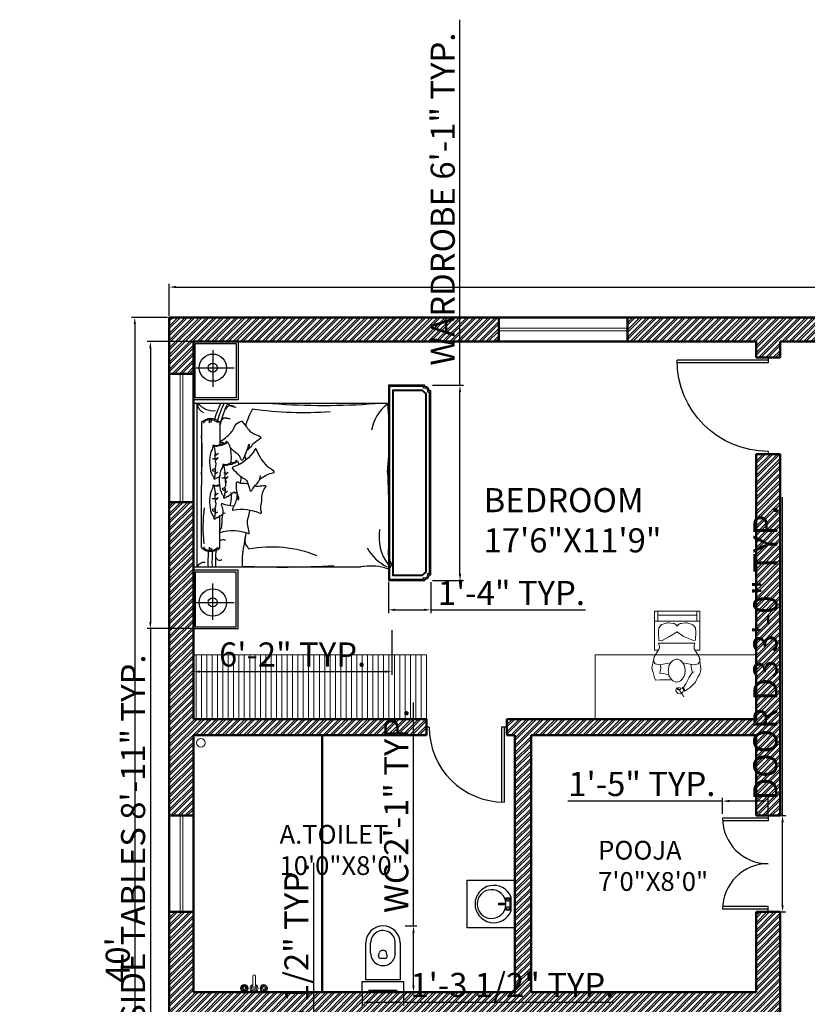
# Model space of a CAD drawing. Units: inches. Extents: x 3590 to 5167, y 65 to 1917.
# Tile 18 of 100: x 3590 to 3884, y 1549 to 1917. Entities that reach past the tile are written whole.
import ezdxf

# ---------------------------------------------------------------- set-up
doc = ezdxf.new("R2010")
doc.units = ezdxf.units.IN
for name, color, linetype, lineweight in [('A-ANNO-DIMS', 2, 'Continuous', 18), ('A-AREA-IDEN', 7, 'Continuous', 18), ('A-DOOR', 3, 'Continuous', 25), ('A-FLOR-FIXT', 8, 'Continuous', 18), ('A-FURN', 21, 'Continuous', 18), ('A-GLAZ', 4, 'Continuous', 18), ('A-WALL', 7, 'Continuous', 50), ('A-WALL-PATT', 251, 'Continuous', 13)]:
    doc.layers.add(name, color=color, linetype=linetype, lineweight=lineweight)
for name, color, linetype in [('FUR', 42, 'Continuous'), ('HA-FUR', 8, 'Continuous'), ('HA-P', 8, 'Continuous'), ('SAN', 5, 'Continuous'), ('SANTEH', 7, 'Continuous'), ('wood', 26, 'Continuous')]:
    doc.layers.add(name, color=color, linetype=linetype)
doc.styles.get("Standard").update_dxf_attribs({"font": 'arial.ttf'})
doc.dimstyles.new('ISO-25', dxfattribs={"dimtxt": 9, "dimasz": 2.5, "dimexe": 1.25, "dimexo": 0.625, "dimtad": 1, "dimdec": 1, "dimlunit": 3, "dimtxsty": 'Standard', "dimcen": 2.5, "dimadec": 0, "dimazin": 0, "dimtfac": 1, "dimtdec": 1, "dimtmove": 0, "dimatfit": 3, "dimfxl": 1, "dimarcsym": 0})

# ---------------------------------------------------------------- blocks, each defined once
blk = doc.blocks.new('*D5')
at = {"layer": 'A-ANNO-DIMS', "color": 0, "lineweight": -2, "transparency": 16777216}
for p, q in [((3645.51, 1806.62), (3645.51, 1818.61)), ((3648.01, 1817.36), (4303.01, 1817.36)), ((4305.51, 1806.62), (4305.51, 1818.61))]:
    blk.add_line(p, q, dxfattribs=at)
at = {"layer": 'A-ANNO-DIMS', "color": 0, "transparency": 16777216}
for points in [[(3648.01, 1817.78), (3648.01, 1816.95), (3645.51, 1817.36)], [(4303.01, 1817.78), (4303.01, 1816.95), (4305.51, 1817.36)]]:
    blk.add_solid(points, dxfattribs=at)
at = {"layer": 'Defpoints', "color": 0, "transparency": 16777216}
for p in [(4305.51, 1817.36), (3645.51, 1806), (4305.51, 1806)]:
    blk.add_point(p, dxfattribs=at)
at = {"layer": 'A-ANNO-DIMS', "color": 0, "transparency": 16777216, "insert": (3975.51, 1822.57), "char_height": 9, "attachment_point": 5}
blk.add_mtext("55'", dxfattribs=at)
blk = doc.blocks.new('*D6')
at = {"layer": 'A-ANNO-DIMS', "color": 0, "lineweight": -2, "transparency": 16777216}
for p, q in [((3644.89, 1806), (3631.39, 1806)), ((3632.64, 1803.5), (3632.64, 1328.5)), ((3644.89, 1326), (3631.39, 1326))]:
    blk.add_line(p, q, dxfattribs=at)
at = {"layer": 'A-ANNO-DIMS', "color": 0, "transparency": 16777216}
for points in [[(3632.22, 1803.5), (3633.06, 1803.5), (3632.64, 1806)], [(3632.22, 1328.5), (3633.06, 1328.5), (3632.64, 1326)]]:
    blk.add_solid(points, dxfattribs=at)
at = {"layer": 'Defpoints', "color": 0, "transparency": 16777216}
for p in [(3645.51, 1806), (3632.64, 1326), (3645.51, 1326)]:
    blk.add_point(p, dxfattribs=at)
at = {"layer": 'A-ANNO-DIMS', "color": 0, "transparency": 16777216, "insert": (3627.42, 1566), "char_height": 9, "attachment_point": 5, "rotation": 90}
blk.add_mtext("40'", dxfattribs=at)
blk = doc.blocks.new('D1')
for p, q in [((1, 0), (1, 34)), ((2, 0), (2, 33.99)), ((0, 0), (2, 0)), ((35, 0), (36, 0))]:
    blk.add_line(p, q)
at = {"ltscale": 0.5}
blk.add_arc((1, 0), 34, 0, 90, dxfattribs=at)
blk = doc.blocks.new('D2')
for p, q in [((1, 0), (1, 28)), ((2, 0), (2, 27.98)), ((0, 0), (2, 0)), ((29, 0), (30, 0))]:
    blk.add_line(p, q)
at = {"ltscale": 0.5}
blk.add_arc((1, 0), 28, 0, 90, dxfattribs=at)
blk = doc.blocks.new('D3')
for p, q in [((1, 0), (1, 17)), ((2, 0), (2, 16.97)), ((34, 0), (34, 16.97)), ((35, 0), (35, 17)), ((0, 0), (2, 0)), ((36, 0), (34, 0))]:
    blk.add_line(p, q)
at = {"ltscale": 0.5}
for centre, start, end in [((1, 0), 0, 90), ((35, 0), 90, 180)]:
    blk.add_arc(centre, 17, start, end, dxfattribs=at)
blk = doc.blocks.new('Faucet - Bathroom top')
for p, q in [((-4.107, 0.125), (-4.375, 0.125)), ((-3.75, 0.4788), (-3.75, 0.75)), ((-3.5, 0.482), (-3.5, 0.75)), ((-3.1461, 0.125), (-2.875, 0.125)), ((3.143, 0.125), (2.875, 0.125)), ((3.5, 0.4788), (3.5, 0.75)), ((3.75, 0.482), (3.75, 0.75)), ((4.1039, 0.125), (4.375, 0.125)), ((-4.1039, -0.125), (-4.375, -0.125)), ((-3.75, -0.4821), (-3.75, -0.75)), ((-3.5, -0.4789), (-3.5, -0.75)), ((-3.143, -0.125), (-2.875, -0.125)), ((-0.5, -0.8639), (-0.5, -4.5)), ((0.5, -4.5), (0.5, -0.8631)), ((3.1461, -0.125), (2.875, -0.125)), ((3.5, -0.4821), (3.5, -0.75)), ((3.75, -0.4789), (3.75, -0.75)), ((4.107, -0.125), (4.375, -0.125))]:
    blk.add_line(p, q)
for centre, radius in [((-3.625, 0), 1.375), ((-4.625, 0), 0.2795), ((-3.625, 0), 0.5), ((-3.625, 1), 0.2795), ((-2.625, 0), 0.2795), ((0, 0), 0.5), ((3.625, 0), 1.375), ((2.625, 0), 0.2795), ((3.625, 0), 0.5), ((3.625, 1), 0.2795), ((4.625, 0), 0.2795), ((-3.625, -1), 0.2795), ((3.625, -1), 0.2795)]:
    blk.add_circle(centre, radius)
for centre, radius, start, end in [((-3.625, 0), 1, 105.2407, 164.2093), ((-3.625, 0), 1, 16.44125, 74.07887), ((0, 0), 1.5, 289.6514, 250.3603), ((0, 0), 1, 300.3431, 239.7554), ((3.625, 0), 1, 106.12, 164.0884), ((3.625, 0), 1, 16.23422, 73.90469), ((-3.625, 0), 1, 196.2342, 253.9047), ((-3.625, 0), 1, 286.12, 344.0884), ((3.625, 0), 1, 196.4413, 254.0789), ((3.625, 0), 1, 285.2407, 344.2093), ((0, -4.5), 0.5, 180, 0)]:
    blk.add_arc(centre, radius, start, end)
blk = doc.blocks.new('y3')
at = {"layer": 'SANTEH', "ltscale": 5}
for p, q in [((38, 131), (38, 521)), ((88, 411), (88, 521)), ((347, 426), (348, 521)), ((398, 521), (398, 131)), ((172, 385), (181, 421)), ((263, 385), (254, 421)), ((244, 358), (191, 358)), ((398, 131), (38, 131)), ((67, 21), (367, 21))]:
    blk.add_line(p, q, dxfattribs=at)
blk.add_lwpolyline([(0, 115), (435, 115), (435, 0), (0, 0), (0, 115)], dxfattribs=at)
for centre, radius, start, end in [((218, 521), 180, 0, 180), ((218, 521), 130, 359.1579, 180), ((218, 411), 130, 180, 5.9855), ((218, 400), 42.2, 30.5234, 149.4766), ((191, 378), 20, 160.5038, 270), ((244, 378), 20, 270, 19.4962)]:
    blk.add_arc(centre, radius, start, end, dxfattribs=at)
blk = doc.blocks.new('r11')
at = {"layer": 'SANTEH', "ltscale": 5}
for p, q in [((0, 0), (600, 0)), ((0, -600), (0, 0)), ((600, 0), (600, -600)), ((210, -50), (390, -50)), ((210, -50), (210, -50)), ((224, -63), (376, -63)), ((224, -113), (224, -63)), ((376, -113), (224, -113)), ((233, -79), (249, -69)), ((233, -98), (233, -79)), ((249, -107), (233, -98)), ((249, -69), (266, -79)), ((266, -98), (249, -107)), ((266, -79), (266, -98)), ((288, -202), (288, -113)), ((312, -113), (312, -202)), ((334, -79), (351, -69)), ((334, -98), (334, -79)), ((351, -107), (334, -98)), ((351, -69), (367, -79)), ((367, -98), (351, -107)), ((367, -79), (367, -98)), ((376, -63), (376, -113)), ((312, -184), (288, -184)), ((312, -202), (288, -202)), ((600, -600), (0, -600))]:
    blk.add_line(p, q, dxfattribs=at)
for centre, radius, start, end in [((300, -266), 234, 112.5, 67.5), ((300, -293), 180, 93.8183, 86.1817)]:
    blk.add_arc(centre, radius, start, end, dxfattribs=at)
blk = doc.blocks.new('A$C0A42580C')
at = {"layer": 'SAN'}
for p, q in [((0.287, 0.03), (0.287, 0.448)), ((2.868, 0.03), (2.868, 0.448)), ((0.095, 0.213), (0.496, 0.213)), ((3.06, 0.213), (2.659, 0.213))]:
    blk.add_line(p, q, dxfattribs=at)
for centre, radius in [((0.287, 0.213), 0.15), ((2.868, 0.213), 0.15), ((0.287, 0.213), 0.05), ((2.868, 0.213), 0.05)]:
    blk.add_circle(centre, radius, dxfattribs=at)
at = {"layer": 'wood'}
for p, q in [((0.678, 0.885), (0.678, 2.139)), ((2.478, 0.802), (2.478, 1.838)), ((2.478, 0), (2.478, 0.802)), ((1.5, 0.342), (1.502, 0.314)), ((1.663, 0.344), (1.643, 0.376)), ((0.888, 0.289), (1.133, 0.289)), ((1.291, 0.235), (1.292, 0.207)), ((1.454, 0.236), (1.434, 0.268)), ((1.729, 0.235), (1.73, 0.207)), ((1.892, 0.236), (1.872, 0.268)), ((2.267, 0.289), (1.916, 0.289)), ((0.678, 0.039), (2.478, 0.039)), ((0.891, 0.089), (1.578, 0.089)), ((2.264, 0.089), (1.578, 0.089)), ((0.678, 0), (2.478, 0))]:
    blk.add_line(p, q, dxfattribs=at)
blk.add_lwpolyline([(0.678, 0), (0.678, 0.885)], dxfattribs=at)
for points in [[(1.516, 0.729, -0.128392), (1.44, 0.883, 0.70791), (1.427, 0.886, -0.16964), (1.185, 0.692, 0.664036), (1.184, 0.678, -0.184649), (1.382, 0.433, 0.662242), (1.397, 0.431, 0.078539), (1.514, 0.567, -0.1736), (1.548, 0.595, -0.02159), (1.636, 0.621, 0.697276), (1.638, 0.641, -0.093019), (1.561, 0.699, 0.216632), (1.472, 0.737, -2.511293)], [(1.68, 0.482, 0.263265), (1.719, 0.484, -0.026108), (1.743, 0.497, 0.027613), (1.714, 0.476, -0.089259), (1.84, 0.429, 0.662242), (1.853, 0.438, -0.162037), (1.888, 0.732, 0.676499), (1.873, 0.748, -0.160513), (1.79, 0.744, 0.07473), (1.72, 0.752, -0.187721), (1.597, 0.796, 0.70791), (1.585, 0.789, -0.010003), (1.592, 0.714, -0.07079), (1.589, 0.672, 0.099539)], [(1.121, 0.345, 0.032543), (1.109, 0.309, -0.658965), (1.092, 0.306, 0.074753), (0.989, 0.423, 0.100988), (0.953, 0.443, -0.270711), (0.875, 0.527, -0.276825), (0.877, 0.534, -0.014937), (0.97, 0.608, 0.134834), (1.013, 0.664, -0.023706), (1.047, 0.737, -0.664036), (1.062, 0.739, -0.035987), (1.119, 0.663, 0.118631), (1.141, 0.641, -0.132738), (1.196, 0.586)], [(1.176, 0.593, 0.013884), (1.155, 0.613, 0.174178), (1.144, 0.618, 0.104076), (1.136, 0.616, 0.389829), (1.132, 0.61, 0.296089), (1.141, 0.602, -0.036701), (1.157, 0.599, -0.040547), (1.302, 0.543, -0.70791), (1.302, 0.53, -0.016811), (1.263, 0.509, 0.11866), (1.241, 0.49, -0.048791), (1.165, 0.405, 0.103757)], [(1.567, 0.601, 0.057807), (1.561, 0.534, -0.173425), (1.546, 0.49, 0.589988), (1.554, 0.471, 0.137312), (1.724, 0.499, 0.137312)], [(1.811, 0.445, -0.069098), (1.783, 0.319, 0.658965), (1.796, 0.306, -0.049789), (1.852, 0.323, -0.103757), (1.89, 0.323, 0.055725), (2.02, 0.31, -0.11866), (2.048, 0.304, 0.016811), (2.088, 0.286, 0.70791), (2.099, 0.294, -0.16964), (2.11, 0.604, 0.664036), (2.1, 0.614, 0.023706), (2.021, 0.597, -0.134834), (1.95, 0.598, 0.012748), (1.852, 0.623)], [(1.311, 0.476, 0.145733), (1.307, 0.468, 0.488583), (1.309, 0.466, -0.012138), (1.313, 0.466, -0.125673), (1.321, 0.465, -0.750706)], [(1.315, 0.475, -0.274893), (1.338, 0.453, 0.051436), (1.347, 0.429, -0.086628), (1.353, 0.408, 0.040196), (1.359, 0.377, -0.184744), (1.356, 0.334, -2.554464)], [(1.317, 0.468, -0.060098), (1.328, 0.457, -0.16247), (1.331, 0.449, 0.120018), (1.349, 0.381, -0.060072), (1.354, 0.369, -0.13107), (1.354, 0.339, -0.024415), (1.353, 0.337, 0.070398), (1.35, 0.323, 0.528689), (1.352, 0.322, -0.069388), (1.356, 0.322, -0.158233), (1.407, 0.306, 0.085461), (1.425, 0.298, 0.147196), (1.657, 0.304, 0.10985), (1.682, 0.319, -0.179095), (1.713, 0.332, -2.318897)], [(1.101, 0.369, 0.145733), (1.097, 0.36, 0.488583), (1.099, 0.358, -0.012138), (1.104, 0.359, -0.125673), (1.112, 0.357, -0.750706)], [(1.106, 0.368, -0.274893), (1.128, 0.345, 0.051436), (1.137, 0.322, -0.086628), (1.144, 0.3, 0.040196), (1.15, 0.27, -0.184744), (1.146, 0.227, -2.554464)], [(1.108, 0.361, -0.060098), (1.119, 0.35, -0.16247), (1.122, 0.341, 0.120018), (1.14, 0.274, -0.060072), (1.145, 0.262, -0.13107), (1.145, 0.232, -0.024415), (1.144, 0.23, 0.070398), (1.141, 0.216, 0.528689), (1.143, 0.214, -0.069388), (1.146, 0.215, -0.158233), (1.198, 0.199, 0.085461), (1.216, 0.191, 0.147196), (1.448, 0.197, 0.10985), (1.473, 0.212, -0.179095), (1.503, 0.224, -2.318897)], [(1.351, 0.322, -0.117141), (1.369, 0.335, -0.025084), (1.453, 0.348, 0.033691)], [(1.436, 0.38, -0.198519), (1.452, 0.349, 0.826402), (1.456, 0.349, 0.095956), (1.456, 0.353, 0.242899), (1.446, 0.369, -17.523452)], [(1.545, 0.353, -0.083557), (1.507, 0.355, 0.203162), (1.485, 0.379, -0.208037), (1.504, 0.341, 0.124669), (1.443, 0.347, 0.965934)], [(1.539, 0.369, 0.145733), (1.536, 0.36, 0.488583), (1.538, 0.358, -0.012138), (1.542, 0.359, -0.125673), (1.55, 0.357, -0.750706)], [(1.545, 0.353, -0.008229), (1.573, 0.352, 0.033691)], [(1.573, 0.352, -0.46905), (1.615, 0.321, 0.420988), (1.62, 0.317, 0.857652), (1.622, 0.348, 0.548526)], [(1.603, 0.345, -0.099719), (1.622, 0.348, 0.102691)], [(1.621, 0.349, -0.010168), (1.656, 0.345, 0.033691), (1.691, 0.342, -0.220869), (1.715, 0.331, -0.288972)], [(1.141, 0.214, -0.117141), (1.159, 0.227, -0.025084), (1.244, 0.24, 0.033691)], [(1.227, 0.273, -0.198519), (1.243, 0.242, 0.826402), (1.246, 0.241, 0.095956), (1.247, 0.245, 0.242899), (1.237, 0.261, -17.523452)], [(1.335, 0.245, -0.083557), (1.298, 0.247, 0.203162), (1.276, 0.272, -0.208037), (1.295, 0.233, 0.124669), (1.234, 0.239, 0.965934)], [(1.335, 0.245, -0.008229), (1.363, 0.244, 0.033691)], [(1.363, 0.244, -0.46905), (1.406, 0.213, 0.420988), (1.411, 0.209, 0.857652), (1.413, 0.241, 0.548526)], [(1.394, 0.237, -0.099719), (1.413, 0.241, 0.102691)], [(1.412, 0.241, -0.010168), (1.446, 0.237, 0.033691), (1.481, 0.235, -0.220869), (1.505, 0.224, -0.288972)], [(1.572, 0.286, 0.022869), (1.578, 0.274, -0.060072), (1.583, 0.262, -0.13107), (1.583, 0.232, -0.024415), (1.582, 0.23, 0.070398), (1.579, 0.216, 0.528689), (1.581, 0.214, -0.069388), (1.584, 0.215, -0.158233), (1.636, 0.199, 0.085461), (1.654, 0.191, 0.147196), (1.886, 0.197, 0.10985), (1.911, 0.212, -0.179095), (1.941, 0.224, -2.318897)], [(1.58, 0.214, -0.117141), (1.597, 0.227, -0.025084), (1.682, 0.24, 0.033691)], [(1.584, 0.287, 0.023398), (1.588, 0.27, -0.184744), (1.584, 0.227, -2.554464)], [(1.665, 0.273, -0.198519), (1.681, 0.242, 0.826402), (1.684, 0.241, 0.095956), (1.685, 0.245, 0.242899), (1.675, 0.261, -17.523452)], [(1.773, 0.245, -0.083557), (1.736, 0.247, 0.203162), (1.714, 0.272, -0.208037), (1.733, 0.233, 0.124669), (1.672, 0.239, 0.965934)], [(1.773, 0.245, -0.008229), (1.801, 0.244, 0.033691)], [(1.801, 0.244, -0.46905), (1.844, 0.213, 0.420988), (1.849, 0.209, 0.857652), (1.851, 0.241, 0.548526)], [(1.832, 0.237, -0.099719), (1.851, 0.241, 0.102691)], [(1.85, 0.241, -0.010168), (1.885, 0.237, 0.033691), (1.919, 0.235, -0.220869), (1.943, 0.224, -0.288972)]]:
    blk.add_lwpolyline(points, format="xyb", dxfattribs=at)
for points in [[(0.64, 0), (0, 0), (0, 0.49), (0.64, 0.49)], [(0.62, 0.02), (0.02, 0.02), (0.02, 0.47), (0.62, 0.47)], [(2.515, 0), (3.155, 0), (3.155, 0.49), (2.515, 0.49)], [(2.535, 0.02), (3.135, 0.02), (3.135, 0.47), (2.535, 0.47)]]:
    blk.add_lwpolyline(points, close=True, dxfattribs=at)
for centre, radius, start, end in [((2.312, 2.383), 0.244, 254.1515, 300.9557), ((2.45, 2.131), 0.0445, 324.1895, 118.922), ((1.034, -2.14), 4.292, 84.5608, 94.7164), ((1.049, 2.403), 0.451, 217.4794, 260.3599), ((2.021, -11.079), 13.229, 88.7555, 92.5113), ((2.149, 2.547), 0.508, 260.6549, 306.4415), ((2.017, 2.357), 0.513, 299.0817, 333.4437), ((3.137, 1.95), 0.669, 166.6404, 189.6571), ((-7.084, 1.433), 7.786, 355.8482, 4.1518), ((-7.244, 0.994), 9.723, 357.3447, 3.2307), ((-3.167, 1.214), 3.947, 351.7729, 4.1839), ((3.58, 0.862), 1.321, 157.813, 191.1515), ((1.161, 1.418), 0.877, 241.2136, 254.4188), ((1.258, 0.636), 0.0695, 238.5892, 301.9267), ((1.786, -2.16), 2.756, 80.8988, 83.4666), ((2.181, 0.686), 0.122, 247.3775, 321.1316), ((2.419, 1.382), 0.846, 255.7754, 273.2559), ((0.59, 0.469), 0.13, 317.3822, 359.7039), ((0.772, 0.413), 0.0674, 147.6823, 245.7987), ((1.355, 0.447), 0.0529, 114.2128, 146.154), ((2.613, -2.35), 3.12, 113.8318, 114.2128), ((1.471, 0.072), 0.453, 80.624, 88.7406), ((1.403, -0.339), 0.869, 79.7149, 80.624), ((1.63, 0.454), 0.0342, 31.141, 54.9542), ((1.671, 0.449), 0.0156, 131.9623, 212.0813), ((1.673, 0.442), 0.0178, 140.4179, 157.6327), ((1.723, 0.482), 0.0777, 212.0813, 227.364), ((1.566, 0.415), 0.109, 24.2099, 31.141), ((1.664, 0.45), 0.00568, 95.5225, 140.4179), ((1.663, 0.459), 0.00309, 275.5225, 24.2099), ((1.161, 1.319), 1.057, 242.7667, 257.104), ((1.161, 1.319), 1.094, 243.7555, 254.4906), ((0.031, 0.458), 0.817, 350.4237, 356.2506), ((0.902, 0.356), 0.0605, 155.8342, 254.4106), ((1.145, 0.339), 0.0529, 114.2128, 146.154), ((2.403, -2.458), 3.12, 113.5569, 114.2128), ((1.205, 0.291), 0.121, 99.4203, 113.5569), ((1.277, -0.148), 0.566, 95.9038, 99.4203), ((1.263, -0.005), 0.422, 88.7406, 95.9038), ((1.262, -0.035), 0.453, 80.624, 88.7406), ((1.194, -0.446), 0.869, 79.4587, 80.624), ((1.421, 0.346), 0.0342, 31.141, 54.9542), ((1.461, 0.341), 0.0156, 131.9623, 212.0813), ((1.463, 0.335), 0.0178, 140.4179, 157.6327), ((1.357, 0.308), 0.109, 24.2099, 31.141), ((1.454, 0.342), 0.00568, 95.5225, 140.4179), ((1.453, 0.351), 0.00309, 275.5225, 24.2099), ((1.701, -0.005), 0.422, 88.7406, 95.9038), ((1.639, 0.39), 0.0469, 17.3262, 47.364), ((1.711, 0.413), 0.028, 197.3262, 226.173), ((1.643, 0.342), 0.0695, 26.6176, 46.173), ((1.82, 0.431), 0.129, 206.6176, 215.9619), ((1.7, -0.035), 0.453, 80.624, 88.7406), ((1.715, 0.335), 0.00379, 207.1817, 328.0298), ((1.697, 0.342), 0.023, 350.7643, 35.9619), ((1.706, 0.341), 0.0145, 328.0298, 350.7643), ((1.632, -0.446), 0.869, 78.4392, 80.624), ((1.902, 0.335), 0.0178, 140.4179, 157.6327), ((1.952, 0.374), 0.0777, 212.0813, 227.364), ((1.892, 0.342), 0.00568, 95.5225, 140.4179), ((2.251, 0.326), 0.071, 155.8684, 211.0451), ((0.529, 0.224), 0.231, 309.6305, 4.2746), ((1.161, 1.282), 1.094, 243.7555, 254.3893), ((0.985, 0.19), 0.138, 134.3928, 227.2375), ((0.999, 0.173), 0.143, 136.5824, 164.9725), ((1.501, 0.305), 0.028, 197.3262, 226.173), ((1.434, 0.235), 0.0695, 26.6176, 46.173), ((1.611, 0.323), 0.129, 206.6176, 215.9619), ((1.506, 0.227), 0.00379, 207.1817, 328.0298), ((1.488, 0.234), 0.023, 350.7643, 35.9619), ((1.496, 0.233), 0.0145, 328.0298, 350.7643), ((1.868, 0.283), 0.0469, 17.3262, 47.364), ((1.939, 0.305), 0.028, 197.3262, 226.173), ((1.872, 0.235), 0.0695, 26.6176, 46.173), ((2.049, 0.323), 0.129, 206.6176, 215.9619), ((1.944, 0.227), 0.00379, 207.1817, 328.0298), ((1.926, 0.234), 0.023, 350.7643, 35.9619), ((1.935, 0.233), 0.0145, 328.0298, 350.7643), ((2.156, 0.173), 0.143, 15.0275, 43.4176), ((2.17, 0.19), 0.138, 312.7625, 45.6072), ((2.419, 1.267), 1.026, 263.0903, 273.2559), ((2.362, 0.291), 0.0419, 290.7858, 35.3631), ((0.673, 0.151), 0.113, 279.2382, 338.7382), ((0.87, 0.179), 0.0229, 77.149, 159.1786), ((0.88, 0.137), 0.0592, 81.4779, 123.1193), ((0.841, 0.185), 0.0128, 299.4706, 57.4442), ((0.84, 0.185), 0.0112, 314.8966, 45.1034), ((0.884, 0.229), 0.0569, 229.7059, 281.1153), ((0.947, 0.177), 0.0862, 185.5372, 234.6869), ((2.045, 1.702), 1.598, 262.1364, 276.4879), ((2.208, 0.177), 0.0862, 305.3131, 354.4628), ((2.271, 0.229), 0.0569, 258.8847, 310.2941), ((2.275, 0.137), 0.0592, 56.8807, 98.5221), ((2.285, 0.179), 0.0229, 20.8214, 102.851), ((2.419, 1.222), 1.063, 263.2362, 273.2559), ((2.314, 0.185), 0.0128, 122.5558, 240.5294), ((2.315, 0.185), 0.0112, 134.8966, 225.1034), ((2.419, 1.267), 1.063, 263.9437, 273.2559), ((2.508, 0.115), 0.0792, 169.9467, 248.2401), ((1.248, -2.592), 2.689, 85.4722, 94.5278)]:
    blk.add_arc(centre, radius, start, end, dxfattribs=at)
blk = doc.blocks.new('A$C623F1DA0')
at = {"layer": 'FUR'}
blk.add_lwpolyline([(0.628, 2.912, 0.414214), (0.562, 2.978), (0.562, 3), (0, 3), (0, 0), (0.562, 0), (0.562, 0.022, 0.414214), (0.628, 0.088), (0.65, 0.088), (0.65, 2.912)], format="xyb", close=True, dxfattribs=at)
at = {"layer": 'HA-FUR'}
blk.add_lwpolyline([(0.603, 2.892, 0.710288), (0.542, 2.953), (0.542, 2.98), (0.02, 2.98), (0.02, 0.02), (0.542, 0.02), (0.542, 0.047, 0.710288), (0.603, 0.108), (0.63, 0.108), (0.63, 2.892)], format="xyb", close=True, dxfattribs=at)
at = {"layer": 'HA-P'}
for points in [[(0.07, 2.93), (0.521, 2.93), (0.58, 2.871), (0.58, 0.129), (0.521, 0.07), (0.07, 0.07)], [(0.08, 2.92), (0.517, 2.92), (0.57, 2.867), (0.57, 0.133), (0.517, 0.08), (0.08, 0.08)]]:
    blk.add_lwpolyline(points, close=True, dxfattribs=at)
blk = doc.blocks.new('DESK-CHAIR')
for p, q in [((3674.9, 1522.4), (3674.54, 1520.79)), ((3675.51, 1522.74), (3674.9, 1522.4)), ((3680.2, 1521.08), (3677.49, 1522.71)), ((3694.59, 1522.58), (3680.09, 1522.58)), ((3680.09, 1522.58), (3680.09, 1521.15)), ((3694.59, 1505.74), (3694.59, 1522.58)), ((3674.54, 1520.79), (3675.25, 1516.67)), ((3682.6, 1521.15), (3681.85, 1520.9)), ((3682.6, 1521.15), (3682.6, 1507.53)), ((3682.6, 1507.53), (3682.6, 1521.15)), ((3683.49, 1520.07), (3683.66, 1520.91)), ((3685.1, 1517.02), (3683.49, 1520.07)), ((3683.73, 1520.97), (3686.72, 1521.15)), ((3686.72, 1521.15), (3688.33, 1520.97)), ((3688.33, 1520.97), (3689.58, 1520.07)), ((3689.58, 1520.07), (3690.17, 1518.15)), ((3686.89, 1514.16), (3685.1, 1517.02)), ((3690.24, 1517.32), (3690.04, 1515.67)), ((3664.74, 1511.43), (3666.04, 1512.26)), ((3665.07, 1511.29), (3664.74, 1511.43)), ((3664.84, 1511.19), (3666.07, 1511.86)), ((3666.04, 1512.26), (3666.24, 1511.79)), ((3666.07, 1511.86), (3667.43, 1510.93)), ((3674.54, 1507.89), (3675.25, 1512.01)), ((3683.67, 1508.07), (3685.1, 1511.83)), ((3685.1, 1511.83), (3686.89, 1514.16)), ((3689.31, 1514.37), (3689.04, 1514.16)), ((3689.31, 1513.95), (3689.04, 1514.16)), ((3690.24, 1511), (3690.04, 1512.64)), ((3666.04, 1509.36), (3664.84, 1511.19)), ((3668.13, 1507.37), (3666.04, 1509.36)), ((3667.43, 1510.93), (3669.7, 1509.83)), ((3669.7, 1509.83), (3671.06, 1508.9)), ((3671.06, 1508.9), (3671.66, 1508.47)), ((3671.66, 1508.47), (3671.96, 1507.77)), ((3674.9, 1506.27), (3674.54, 1507.89)), ((3680.2, 1507.6), (3677.49, 1505.97)), ((3682.6, 1507.53), (3681.85, 1507.78)), ((3683.8, 1507.4), (3683.67, 1508.07)), ((3688.33, 1507.35), (3689.03, 1507.86)), ((3689.78, 1508.89), (3690.17, 1510.17)), ((3670.06, 1506.4), (3668.13, 1507.37)), ((3677.49, 1505.97), (3673.14, 1505.31)), ((3675.51, 1505.94), (3674.9, 1506.27)), ((3680.09, 1507.53), (3680.09, 1505.74)), ((3680.09, 1505.74), (3694.59, 1505.74)), ((3683.88, 1507.34), (3686.72, 1507.17)), ((3686.72, 1507.17), (3688.33, 1507.35))]:
    blk.add_line(p, q)
for points in [[(3677.49, 1522.71), (3673.28, 1523.65), (3671.67, 1523.12), (3669.7, 1522.58), (3668.81, 1522.22), (3668.99, 1520.61), (3668.99, 1519), (3668.99, 1516.67)], [(3664.74, 1511.43), (3664.42, 1512.05), (3663.77, 1512.78), (3663.87, 1513.9), (3664.88, 1514.67), (3665.92, 1514.37), (3665.9, 1514.02), (3665.32, 1514.02), (3665.3, 1513.1), (3665.82, 1512.66), (3666.07, 1513.84)], [(3671.66, 1508.47), (3672.6, 1508.69), (3673.82, 1508.93), (3674.7, 1508.93)], [(3670.06, 1506.4), (3671.04, 1505.75), (3672.02, 1505.46), (3672.8, 1505.31), (3673.24, 1505.31)]]:
    blk.add_lwpolyline(points)
at = {"const_width": 0.39}
blk.add_lwpolyline([(3666.01, 1513.98), (3662.61, 1511.61)], dxfattribs=at)
for centre, radius, start, end in [((3676.47, 1521), 1.98, 59.0235, 119.0669), ((3681.22, 1522.78), 1.98, 239.0235, 288.4436), ((3683.74, 1520.89), 0.0779, 93.3682, 168.6956), ((3683.74, 1520.89), 0.0779, 93.3682, 168.6956), ((3688.07, 1515.92), 1.98, 308.6739, 352.8785), ((3688.27, 1517.56), 1.98, 352.8785, 17.0946), ((3688.07, 1512.4), 1.98, 7.1215, 51.3261), ((3681.22, 1505.89), 1.98, 71.5564, 120.9765), ((3687.88, 1509.47), 1.98, 305.5514, 342.9054), ((3688.27, 1510.75), 1.98, 342.9054, 7.1215), ((3676.47, 1507.67), 1.98, 240.9331, 300.9765), ((3683.88, 1507.42), 0.0779, 191.3044, 266.6318)]:
    blk.add_arc(centre, radius, start, end)
blk = doc.blocks.new('*D286')
at = {"layer": 'A-ANNO-DIMS', "color": 0, "lineweight": -2, "transparency": 16777216}
for p, q in [((3653.89, 1797), (3637.19, 1797)), ((3638.44, 1794.5), (3638.44, 1692.33)), ((3653.89, 1689.83), (3637.19, 1689.83)), ((3638.44, 1689.83), (3638.44, 1475.12))]:
    blk.add_line(p, q, dxfattribs=at)
at = {"layer": 'A-ANNO-DIMS', "color": 0, "transparency": 16777216}
for points in [[(3638.02, 1794.5), (3638.85, 1794.5), (3638.44, 1797)], [(3638.02, 1692.33), (3638.85, 1692.33), (3638.44, 1689.83)]]:
    blk.add_solid(points, dxfattribs=at)
at = {"layer": 'Defpoints', "color": 0, "transparency": 16777216}
for p in [(3654.51, 1797), (3638.44, 1689.83), (3654.51, 1689.83)]:
    blk.add_point(p, dxfattribs=at)
at = {"layer": 'A-ANNO-DIMS', "color": 0, "transparency": 16777216, "insert": (3633.16, 1581.22), "char_height": 9, "attachment_point": 5, "rotation": 90}
blk.add_mtext('BED WITH SIDE TABLES 8\'-11" TYP.', dxfattribs=at)
blk = doc.blocks.new('*D287')
at = {"layer": 'A-ANNO-DIMS', "color": 0, "lineweight": -2, "transparency": 16777216}
for p, q in [((3654.51, 1689.2), (3654.51, 1672.5)), ((3728.56, 1689.2), (3728.56, 1672.5)), ((3657.01, 1673.75), (3726.06, 1673.75))]:
    blk.add_line(p, q, dxfattribs=at)
at = {"layer": 'A-ANNO-DIMS', "color": 0, "transparency": 16777216}
for points in [[(3657.01, 1674.17), (3657.01, 1673.33), (3654.51, 1673.75)], [(3726.06, 1674.17), (3726.06, 1673.33), (3728.56, 1673.75)]]:
    blk.add_solid(points, dxfattribs=at)
at = {"layer": 'Defpoints', "color": 0, "transparency": 16777216}
for p in [(3654.51, 1689.83), (3728.56, 1689.83), (3728.56, 1673.75)]:
    blk.add_point(p, dxfattribs=at)
at = {"layer": 'A-ANNO-DIMS', "color": 0, "transparency": 16777216, "insert": (3691.54, 1678.97), "char_height": 9, "attachment_point": 5}
blk.add_mtext('6\'-2" TYP.', dxfattribs=at)
blk = doc.blocks.new('*D288')
at = {"layer": 'A-ANNO-DIMS', "color": 0, "lineweight": -2, "transparency": 16777216}
for p, q in [((3754.01, 1780.69), (3754.01, 1917.2)), ((3743.7, 1780.69), (3755.26, 1780.69)), ((3754.01, 1710.26), (3754.01, 1778.19)), ((3743.7, 1707.76), (3755.26, 1707.76))]:
    blk.add_line(p, q, dxfattribs=at)
at = {"layer": 'A-ANNO-DIMS', "color": 0, "transparency": 16777216}
for points in [[(3753.59, 1778.19), (3754.43, 1778.19), (3754.01, 1780.69)], [(3753.59, 1710.26), (3754.43, 1710.26), (3754.01, 1707.76)]]:
    blk.add_solid(points, dxfattribs=at)
at = {"layer": 'Defpoints', "color": 0, "transparency": 16777216}
for p in [(3743.07, 1780.69), (3754.01, 1780.69), (3743.07, 1707.76)]:
    blk.add_point(p, dxfattribs=at)
at = {"layer": 'A-ANNO-DIMS', "color": 0, "transparency": 16777216, "insert": (3748.73, 1850.2), "char_height": 9, "attachment_point": 5, "rotation": 90}
blk.add_mtext('WARDROBE 6\'-1" TYP.', dxfattribs=at)
blk = doc.blocks.new('*D289')
at = {"layer": 'A-ANNO-DIMS', "color": 0, "lineweight": -2, "transparency": 16777216}
for p, q in [((3727.27, 1707.13), (3727.27, 1695.57)), ((3743.07, 1707.13), (3743.07, 1695.57)), ((3729.77, 1696.82), (3740.57, 1696.82)), ((3743.07, 1696.82), (3800.83, 1696.82))]:
    blk.add_line(p, q, dxfattribs=at)
at = {"layer": 'A-ANNO-DIMS', "color": 0, "transparency": 16777216}
for points in [[(3729.77, 1697.23), (3729.77, 1696.4), (3727.27, 1696.82)], [(3740.57, 1697.23), (3740.57, 1696.4), (3743.07, 1696.82)]]:
    blk.add_solid(points, dxfattribs=at)
at = {"layer": 'Defpoints', "color": 0, "transparency": 16777216}
for p in [(3727.27, 1707.76), (3743.07, 1707.76), (3743.07, 1696.82)]:
    blk.add_point(p, dxfattribs=at)
at = {"layer": 'A-ANNO-DIMS', "color": 0, "transparency": 16777216, "insert": (3773.2, 1701.96), "char_height": 9, "attachment_point": 5}
blk.add_mtext('1\'-4" TYP.', dxfattribs=at)
blk = doc.blocks.new('*D303')
at = {"layer": 'A-ANNO-DIMS', "color": 0, "lineweight": -2, "transparency": 16777216}
for p, q in [((3699.41, 1523.65), (3699.41, 1602.39)), ((3695.22, 1523.65), (3700.66, 1523.65)), ((3699.41, 1507.81), (3699.41, 1521.15)), ((3695.22, 1505.31), (3700.66, 1505.31))]:
    blk.add_line(p, q, dxfattribs=at)
at = {"layer": 'A-ANNO-DIMS', "color": 0, "transparency": 16777216}
for points in [[(3698.99, 1521.15), (3699.83, 1521.15), (3699.41, 1523.65)], [(3698.99, 1507.81), (3699.83, 1507.81), (3699.41, 1505.31)]]:
    blk.add_solid(points, dxfattribs=at)
at = {"layer": 'Defpoints', "color": 0, "transparency": 16777216}
for p in [(3694.59, 1523.65), (3699.41, 1523.65), (3694.59, 1505.31)]:
    blk.add_point(p, dxfattribs=at)
at = {"layer": 'A-ANNO-DIMS', "color": 0, "transparency": 16777216, "insert": (3694.13, 1564.27), "char_height": 9, "attachment_point": 5, "rotation": 90}
blk.add_mtext('1\'-6 1/2" TYP.', dxfattribs=at)
blk = doc.blocks.new('*D304')
at = {"layer": 'A-ANNO-DIMS', "color": 0, "lineweight": -2, "transparency": 16777216}
for p, q in [((3736.66, 1578.79), (3736.66, 1662.21)), ((3733.56, 1578.79), (3737.91, 1578.79)), ((3736.66, 1556.5), (3736.66, 1576.29)), ((3733.56, 1554), (3737.91, 1554))]:
    blk.add_line(p, q, dxfattribs=at)
at = {"layer": 'A-ANNO-DIMS', "color": 0, "transparency": 16777216}
for points in [[(3736.24, 1576.29), (3737.07, 1576.29), (3736.66, 1578.79)], [(3736.24, 1556.5), (3737.07, 1556.5), (3736.66, 1554)]]:
    blk.add_solid(points, dxfattribs=at)
at = {"layer": 'Defpoints', "color": 0, "transparency": 16777216}
for p in [(3732.94, 1578.79), (3736.66, 1578.79), (3732.94, 1554)]:
    blk.add_point(p, dxfattribs=at)
at = {"layer": 'A-ANNO-DIMS', "color": 0, "transparency": 16777216, "insert": (3731.38, 1621.75), "char_height": 9, "attachment_point": 5, "rotation": 90}
blk.add_mtext('WC 2\'-1" TYP.', dxfattribs=at)
blk = doc.blocks.new('*D305')
at = {"layer": 'A-ANNO-DIMS', "color": 0, "lineweight": -2, "transparency": 16777216}
for p, q in [((3717.55, 1553.37), (3717.55, 1549.03)), ((3732.94, 1553.37), (3732.94, 1549.03)), ((3720.05, 1550.28), (3730.44, 1550.28)), ((3732.94, 1550.28), (3811.67, 1550.28))]:
    blk.add_line(p, q, dxfattribs=at)
at = {"layer": 'A-ANNO-DIMS', "color": 0, "transparency": 16777216}
for points in [[(3720.05, 1550.7), (3720.05, 1549.86), (3717.55, 1550.28)], [(3730.44, 1550.7), (3730.44, 1549.86), (3732.94, 1550.28)]]:
    blk.add_solid(points, dxfattribs=at)
at = {"layer": 'Defpoints', "color": 0, "transparency": 16777216}
for p in [(3717.55, 1554), (3732.94, 1554), (3732.94, 1550.28)]:
    blk.add_point(p, dxfattribs=at)
at = {"layer": 'A-ANNO-DIMS', "color": 0, "transparency": 16777216, "insert": (3773.56, 1555.56), "char_height": 9, "attachment_point": 5}
blk.add_mtext('1\'-3 1/2" TYP.', dxfattribs=at)
blk = doc.blocks.new('*D318')
at = {"layer": 'A-ANNO-DIMS', "color": 0, "lineweight": -2, "transparency": 16777216}
for p, q in [((3874.41, 1620), (3874.41, 1738.94)), ((3869.64, 1620), (3875.66, 1620)), ((3874.41, 1586.5), (3874.41, 1617.5)), ((3869.64, 1584), (3875.66, 1584))]:
    blk.add_line(p, q, dxfattribs=at)
at = {"layer": 'A-ANNO-DIMS', "color": 0, "transparency": 16777216}
for points in [[(3874, 1617.5), (3874.83, 1617.5), (3874.41, 1620)], [(3874, 1586.5), (3874.83, 1586.5), (3874.41, 1584)]]:
    blk.add_solid(points, dxfattribs=at)
at = {"layer": 'Defpoints', "color": 0, "transparency": 16777216}
for p in [(3869.01, 1620), (3874.41, 1620), (3869.01, 1584)]:
    blk.add_point(p, dxfattribs=at)
at = {"layer": 'A-ANNO-DIMS', "color": 0, "transparency": 16777216, "insert": (3869.13, 1680.72), "char_height": 9, "attachment_point": 5, "rotation": 90}
blk.add_mtext('DOOR D3 3\'-0" TYP.', dxfattribs=at)
blk = doc.blocks.new('*D319')
at = {"layer": 'A-ANNO-DIMS', "color": 0, "lineweight": -2, "transparency": 16777216}
for p, q in [((3852.01, 1625.4), (3794.25, 1625.4)), ((3852.01, 1620.62), (3852.01, 1626.65)), ((3866.51, 1625.4), (3854.51, 1625.4)), ((3869.01, 1620.62), (3869.01, 1626.65))]:
    blk.add_line(p, q, dxfattribs=at)
at = {"layer": 'A-ANNO-DIMS', "color": 0, "transparency": 16777216}
for points in [[(3854.51, 1625.82), (3854.51, 1624.98), (3852.01, 1625.4)], [(3866.51, 1625.82), (3866.51, 1624.98), (3869.01, 1625.4)]]:
    blk.add_solid(points, dxfattribs=at)
at = {"layer": 'Defpoints', "color": 0, "transparency": 16777216}
for p in [(3852.01, 1625.4), (3852.01, 1620), (3869.01, 1620)]:
    blk.add_point(p, dxfattribs=at)
at = {"layer": 'A-ANNO-DIMS', "color": 0, "transparency": 16777216, "insert": (3821.88, 1630.62), "char_height": 9, "attachment_point": 5}
blk.add_mtext('1\'-5" TYP.', dxfattribs=at)

msp = doc.modelspace()

# ---------------------------------------------------------------- hatches: boundary and pattern name
at = {"layer": 'A-WALL-PATT', "transparency": 33554687}
h = msp.add_hatch(dxfattribs=at)
h.set_pattern_fill('ANSI32', color=256, scale=0.2)
h.paths.add_polyline_path([(3768.51, 1806), (3645.51, 1806), (3645.51, 1785), (3654.51, 1785), (3654.51, 1797), (3671.16, 1797), (3768.51, 1797)])
h.paths.add_polyline_path([(3909.51, 1806), (3816.51, 1806), (3816.51, 1797), (3864.51, 1797), (3864.51, 1791), (3873.51, 1791), (3873.51, 1797), (3909.51, 1797)])
h.paths.add_polyline_path([(4053.51, 1806), (3969.51, 1806), (3969.51, 1797), (4053.51, 1797)])
h.paths.add_polyline_path([(4215.51, 1806), (4113.51, 1806), (4113.51, 1797), (4206.51, 1797), (4206.51, 1791), (4215.51, 1791)])
h.paths.add_polyline_path([(3654.51, 1737), (3645.51, 1737), (3645.51, 1620), (3654.51, 1620), (3654.51, 1650), (3741.51, 1650), (3741.51, 1656), (3654.51, 1656)], flags=17)
h.paths.add_polyline_path([(3873.51, 1755), (3864.51, 1755), (3864.51, 1656), (3771.51, 1656), (3771.51, 1650), (3774.51, 1650), (3774.51, 1554), (3654.51, 1554), (3654.51, 1584), (3645.51, 1584), (3645.51, 1539), (3654.51, 1539), (3654.51, 1545), (3864.51, 1545), (3864.51, 1539), (3873.51, 1539), (3873.51, 1584), (3864.51, 1584), (3864.51, 1554), (3780.51, 1554), (3780.51, 1650), (3864.51, 1650), (3864.51, 1620), (3873.51, 1620)])
h.paths.add_polyline_path([(3654.51, 1491), (3645.51, 1491), (3645.51, 1326), (3810.51, 1326), (3810.51, 1335), (3809.96, 1335), (3654.51, 1335)])
h.paths.add_polyline_path([(3915.51, 1335), (3873.51, 1335), (3873.51, 1352.87), (3873.51, 1422), (3876.51, 1422), (3876.51, 1431), (3864.51, 1431), (3864.51, 1335), (3858.51, 1335), (3858.51, 1326), (3915.51, 1326)])
h.paths.add_polyline_path([(4028.01, 1335), (4002.51, 1335), (4002.51, 1503), (3981.51, 1503), (3981.51, 1494), (3993.51, 1494), (3993.51, 1431), (3921.51, 1431), (3921.51, 1494), (3933.51, 1494), (3933.51, 1503), (3864.51, 1503), (3864.51, 1494), (3912.51, 1494), (3912.51, 1431), (3906.51, 1431), (3906.51, 1422), (3993.51, 1422), (3993.51, 1335), (3951.51, 1335), (3951.51, 1326), (4028.01, 1326)])
h.paths.add_polyline_path([(4203.51, 1335), (4158.51, 1335), (4158.51, 1527), (4194.51, 1527), (4194.51, 1536), (4149.51, 1536), (4149.51, 1335), (4124.01, 1335), (4124.01, 1326), (4203.51, 1326)])
h.paths.add_polyline_path([(4305.51, 1566), (4296.51, 1566), (4296.51, 1536), (4278.64, 1536), (4260.51, 1536), (4260.51, 1527), (4296.51, 1527), (4296.51, 1521), (4305.51, 1521)])
h.paths.add_polyline_path([(4305.51, 1473), (4296.51, 1473), (4296.51, 1335), (4251.51, 1335), (4251.51, 1326), (4305.51, 1326)])
h.paths.add_polyline_path([(4305.51, 1677), (4215.51, 1677), (4215.51, 1743), (4206.51, 1743), (4206.51, 1677), (4149.51, 1677), (4149.51, 1668), (4296.51, 1668), (4296.51, 1638), (4305.51, 1638)])

# ---------------------------------------------------------------- linework, layer by layer
at = {"layer": 'A-FLOR-FIXT'}
msp.add_circle((3657.31, 1647.13), 1.6, dxfattribs=at)
at = {"layer": 'A-FURN'}
for p, q in [((3827.81, 1692.55), (3827.81, 1696.31)), ((3842.4, 1692.55), (3842.4, 1696.31)), ((3843.5, 1692.55), (3826.65, 1692.55)), ((3842.4, 1694.88), (3827.81, 1694.88)), ((3654.51, 1680), (3741.51, 1680)), ((3655.51, 1680), (3655.51, 1656)), ((3657.51, 1680), (3657.51, 1656)), ((3659.51, 1680), (3659.51, 1656)), ((3661.51, 1680), (3661.51, 1656)), ((3663.51, 1680), (3663.51, 1656)), ((3665.51, 1680), (3665.51, 1656)), ((3667.51, 1680), (3667.51, 1656)), ((3669.51, 1680), (3669.51, 1656)), ((3671.51, 1680), (3671.51, 1656)), ((3673.51, 1680), (3673.51, 1656)), ((3675.51, 1680), (3675.51, 1656)), ((3677.51, 1680), (3677.51, 1656)), ((3679.51, 1680), (3679.51, 1656)), ((3681.51, 1680), (3681.51, 1656)), ((3683.51, 1680), (3683.51, 1656)), ((3685.51, 1680), (3685.51, 1656)), ((3687.51, 1680), (3687.51, 1656)), ((3689.51, 1680), (3689.51, 1656)), ((3691.51, 1680), (3691.51, 1656)), ((3693.51, 1680), (3693.51, 1656)), ((3695.51, 1680), (3695.51, 1656)), ((3697.51, 1680), (3697.51, 1656)), ((3699.51, 1680), (3699.51, 1656)), ((3701.51, 1680), (3701.51, 1656)), ((3703.51, 1680), (3703.51, 1656)), ((3705.51, 1680), (3705.51, 1656)), ((3707.51, 1680), (3707.51, 1656)), ((3709.51, 1680), (3709.51, 1656)), ((3711.51, 1680), (3711.51, 1656)), ((3713.51, 1680), (3713.51, 1656)), ((3715.51, 1680), (3715.51, 1656)), ((3717.51, 1680), (3717.51, 1656)), ((3719.51, 1680), (3719.51, 1656)), ((3721.51, 1680), (3721.51, 1656)), ((3723.51, 1680), (3723.51, 1656)), ((3725.51, 1680), (3725.51, 1656)), ((3727.51, 1680), (3727.51, 1656)), ((3729.51, 1680), (3729.51, 1656)), ((3731.51, 1680), (3731.51, 1656)), ((3733.51, 1680), (3733.51, 1656)), ((3735.51, 1680), (3735.51, 1656)), ((3737.51, 1680), (3737.51, 1656)), ((3739.51, 1680), (3739.51, 1656)), ((3741.51, 1680), (3741.51, 1656)), ((3804.47, 1680), (3864.51, 1680)), ((3804.47, 1680), (3804.47, 1656))]:
    msp.add_line(p, q, dxfattribs=at)
msp.add_lwpolyline([(3838.01, 1674.11, 0.07405), (3837.76, 1675.79, 0.084801), (3837.09, 1677.11, 0.106336), (3836.03, 1678.06, 0.128955), (3834.88, 1678.36, 0.128955), (3833.74, 1678.06, 0.106336), (3832.68, 1677.11, 0.084801), (3832.01, 1675.79, 0.07405), (3831.76, 1674.11, 0.07405), (3832.01, 1672.43, 0.084801), (3832.68, 1671.11, 0.106336), (3833.74, 1670.16, 0.128955), (3834.88, 1669.86, 0.128955), (3836.03, 1670.16, 0.106336), (3837.09, 1671.11, 0.084801), (3837.76, 1672.43, 0.07405)], format="xyb", close=True, dxfattribs=at)
msp.add_lwpolyline([(3832.03, 1672.5), (3829.88, 1673.03), (3828.63, 1673.21), (3828.98, 1675), (3828.8, 1676.44)], dxfattribs=at)
at = {"layer": 'A-GLAZ'}
for p, q in [((3816.51, 1802), (3768.51, 1802)), ((3816.51, 1801), (3768.51, 1801)), ((3649.51, 1737), (3649.51, 1785)), ((3650.51, 1737), (3650.51, 1785)), ((3649.51, 1584), (3649.51, 1620)), ((3650.51, 1584), (3650.51, 1620))]:
    msp.add_line(p, q, dxfattribs=at)
at = {"layer": 'A-WALL'}
for p, q in [((3768.51, 1797), (3768.51, 1806)), ((3816.51, 1797), (3816.51, 1806)), ((3654.51, 1797), (3864.51, 1797)), ((3654.51, 1656), (3654.51, 1797)), ((3864.51, 1791), (3864.51, 1797)), ((3873.51, 1791), (3873.51, 1797)), ((3873.51, 1797), (4206.51, 1797)), ((3864.51, 1791), (3873.51, 1791)), ((3654.51, 1785), (3645.51, 1785)), ((3864.51, 1656), (3864.51, 1755)), ((3864.51, 1755), (3873.51, 1755)), ((3873.51, 1620), (3873.51, 1755)), ((3654.51, 1737), (3645.51, 1737)), ((3654.51, 1656), (3741.51, 1656)), ((3741.51, 1650), (3741.51, 1656)), ((3771.51, 1650), (3771.51, 1656)), ((3771.51, 1656), (3864.51, 1656)), ((3654.51, 1650), (3741.51, 1650)), ((3654.51, 1554), (3654.51, 1650)), ((3702.51, 1554), (3702.51, 1650)), ((3771.51, 1650), (3774.51, 1650)), ((3774.51, 1554), (3774.51, 1650)), ((3780.51, 1554), (3780.51, 1650)), ((3780.51, 1650), (3864.51, 1650)), ((3864.51, 1620), (3864.51, 1650)), ((3654.51, 1620), (3645.51, 1620)), ((3864.51, 1620), (3873.51, 1620)), ((3654.51, 1584), (3645.51, 1584)), ((3864.51, 1554), (3864.51, 1584)), ((3864.51, 1584), (3873.51, 1584)), ((3873.51, 1539), (3873.51, 1584)), ((3774.51, 1554), (3654.51, 1554)), ((3864.51, 1554), (3780.51, 1554))]:
    msp.add_line(p, q, dxfattribs=at)
msp.add_lwpolyline([(4305.51, 1677), (4305.51, 1326), (3645.51, 1326), (3645.51, 1806), (4215.51, 1806)], dxfattribs=at)

# ---------------------------------------------------------------- block references
at = {"layer": 'A-DOOR', "xscale": -1, "rotation": 90}
msp.add_blockref('D1', (3869.01, 1791), dxfattribs=at)
at = {"layer": 'A-DOOR'}
for name, p, rotation in [('D2', (3771.51, 1653), 180), ('D3', (3869.01, 1584), 90)]:
    msp.add_blockref(name, p, dxfattribs=dict(at, rotation=rotation))
at = {"layer": 'A-FLOR-FIXT', "xscale": 0.0297800069284724, "yscale": 0.0297800069284724, "zscale": 0.0297800069284724, "rotation": 270}
msp.add_blockref('r11', (3774.51, 1595.88), dxfattribs=at)
at = {"layer": 'A-FLOR-FIXT', "xscale": 0.0353848906415677, "yscale": 0.0353848906415677, "zscale": 0.0353848906415677}
msp.add_blockref('y3', (3717.55, 1554), dxfattribs=at)
at = {"layer": 'A-FLOR-FIXT', "xscale": -1, "rotation": 180}
msp.add_blockref('Faucet - Bathroom top', (3677.14, 1555.5), dxfattribs=at)
at = {"layer": 'A-FURN', "xscale": 33.96864568351422, "yscale": 33.96864568351422, "zscale": 33.96864568351422, "rotation": 270}
msp.add_blockref('A$C0A42580C', (3654.51, 1797), dxfattribs=at)
at = {"layer": 'A-FURN', "xscale": 24.31060204424285, "yscale": 24.31060204424285, "zscale": 24.31060204424285}
msp.add_blockref('A$C623F1DA0', (3727.27, 1707.76), dxfattribs=at)
at = {"layer": 'A-FURN', "rotation": 89.99999999999369}
msp.add_blockref('DESK-CHAIR', (5349.23, -1998.28), dxfattribs=at)

# ---------------------------------------------------------------- texts
at = {"layer": 'A-AREA-IDEN', "attachment_point": 1}
for s, insert, char_height in [('{\\fTimes New Roman|b0|i0|c0|p18;BEDROOM\\P17\'6"X11\'9"}', (3762.81, 1742.28), 9), ('{\\fTimes New Roman|b0|i0|c0|p18;A.TOILET\\P10\'0"X8\'0"}', (3686.68, 1616.47), 7), ('{\\fTimes New Roman|b0|i0|c0|p18;POOJA\\P7\'0"X8\'0"}', (3805.59, 1610.53), 7)]:
    msp.add_mtext_dynamic_manual_height_columns(s, width=67.3508, gutter_width=12.5, heights=[0], dxfattribs=dict(at, insert=insert, char_height=char_height))

# ---------------------------------------------------------------- dimensions: what is measured, and where the dimension line sits
at = {"layer": 'A-ANNO-DIMS'}
for base, p1, p2, angle, text, picture, middle in [((3754.01, 1780.69), (3743.07, 1707.76), (3743.07, 1780.69), 90, 'WARDROBE <> TYP.', '*D288', (3748.73, 1850.2)), ((3638.44, 1689.83), (3654.51, 1797), (3654.51, 1689.83), 270, 'BED WITH SIDE TABLES <> TYP.', '*D286', (3633.16, 1581.22)), ((3874.41, 1620), (3869.01, 1584), (3869.01, 1620), 90, 'DOOR D3 <> TYP.', '*D318', (3869.13, 1680.72)), ((3736.66, 1578.79), (3732.94, 1554), (3732.94, 1578.79), 90, 'WC <> TYP.', '*D304', (3731.38, 1621.75)), ((3852.01, 1625.4), (3869.01, 1620), (3852.01, 1620), 180, '<> TYP.', '*D319', (3821.88, 1630.62)), ((3699.41, 1523.65), (3694.59, 1505.31), (3694.59, 1523.65), 90, '<> TYP.', '*D303', (3694.13, 1564.27))]:
    dim = msp.add_linear_dim(base=base, p1=p1, p2=p2, angle=angle, text=text, dimstyle='ISO-25', override={"dimdec": 1, "dimlfac": 1, "dimrnd": 0, "dimzin": 1, "dimdsep": 46, "dimlunit": 4, "dimfrac": 2}, dxfattribs=at)
    dim.commit()
    dim.dimension.update_dxf_attribs({"geometry": picture, "text_midpoint": middle})
dim = msp.add_linear_dim(base=(4305.51, 1817.36), p1=(3645.51, 1806), p2=(4305.51, 1806), dimstyle='ISO-25', override={"dimclrd": 0, "dimclre": 0, "dimclrt": 0}, dxfattribs=at)
dim.commit()
dim.dimension.update_dxf_attribs({"geometry": '*D5', "text_midpoint": (3975.51, 1822.57)})
dim = msp.add_linear_dim(base=(3632.64, 1326), p1=(3645.51, 1806), p2=(3645.51, 1326), angle=90, dimstyle='ISO-25', override={"dimclrd": 0, "dimclre": 0, "dimclrt": 0}, dxfattribs=at)
dim.commit()
dim.dimension.update_dxf_attribs({"geometry": '*D6', "text_midpoint": (3627.42, 1566)})
for base, p1, p2, picture, middle in [((3743.07, 1696.82), (3727.27, 1707.76), (3743.07, 1707.76), '*D289', (3773.2, 1701.96)), ((3728.56, 1673.7503), (3654.5119, 1689.8262), (3728.56, 1689.8262), '*D287', (3691.5359, 1678.9705)), ((3732.94, 1550.28), (3717.55, 1554), (3732.94, 1554), '*D305', (3773.56, 1555.56))]:
    dim = msp.add_linear_dim(base=base, p1=p1, p2=p2, text='<> TYP.', dimstyle='ISO-25', override={"dimdec": 1, "dimlfac": 1, "dimrnd": 0, "dimzin": 1, "dimdsep": 46, "dimlunit": 4, "dimfrac": 2}, dxfattribs=at)
    dim.commit()
    dim.dimension.update_dxf_attribs({"geometry": picture, "text_midpoint": middle})

doc.saveas('drawing.dxf')
